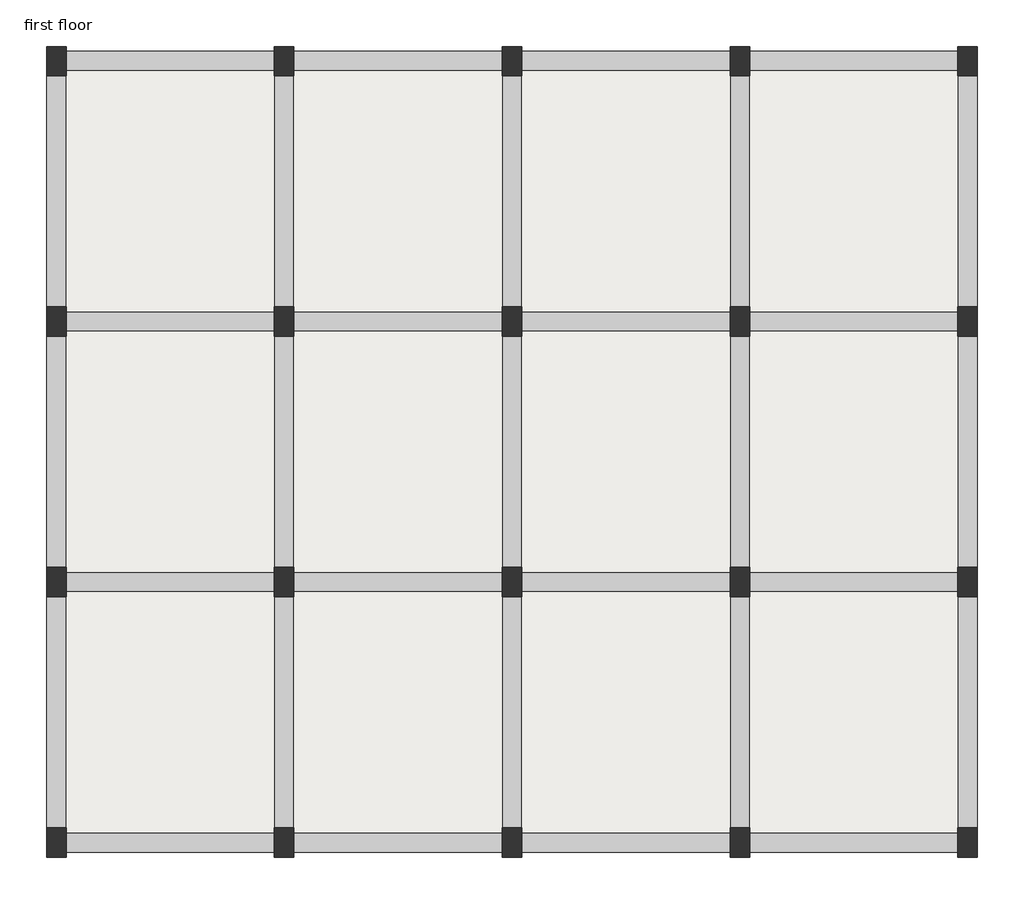
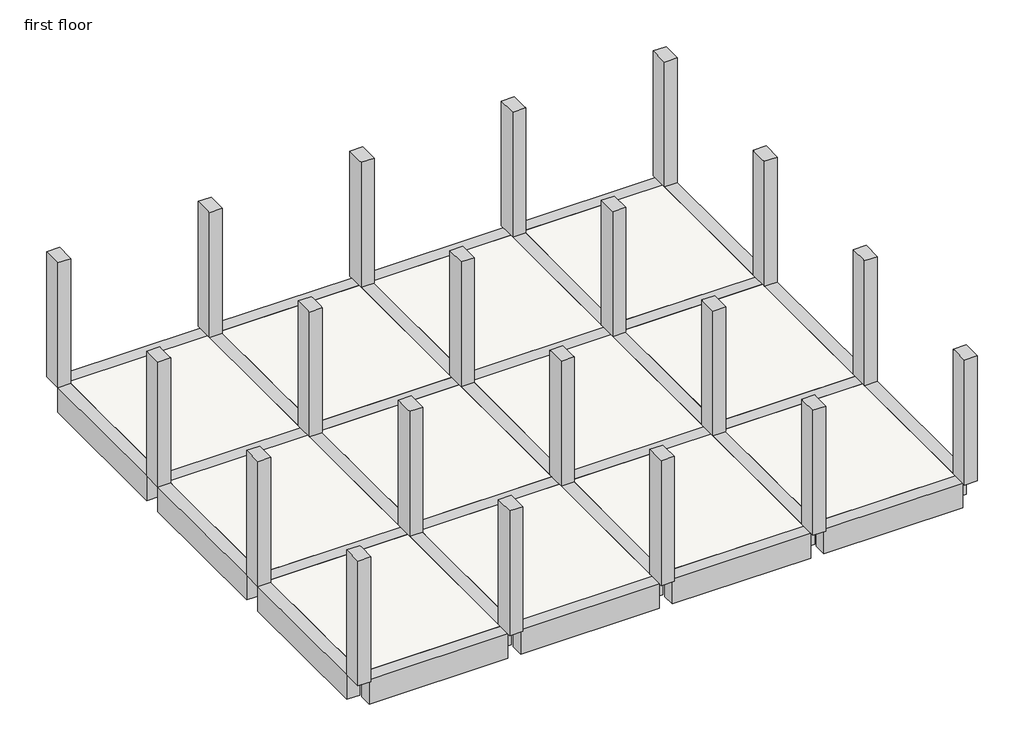
# One storey: 31 beams, 20 columns, 12 slabs.
"""IFC4 building model written with IfcOpenShell, lengths in millimetres."""

from ifc_helpers import new_model, si_unit, frame, origin, place, context, project, spatial, polyline, outline, extrude, faceted_brep, element, save

model = new_model("IFC4")

# Units and contexts
model_context = context("Model", 3, world=origin())
ifc_project = project(units=[si_unit("LENGTHUNIT", "METRE", prefix="MILLI")], contexts=[model_context])

# Site, building, storey
site = spatial("IfcSite", under=ifc_project)
building = spatial("IfcBuilding", under=site)
storey = spatial("IfcBuildingStorey", under=building, Name="first floor", Elevation=3048.0)

# Beams
placement = place(None, origin())
element("IfcBeam", 1, ObjectType="M_Concrete-Rectangular Beam : 300 x 600mm", at=placement, inside=storey, context=model_context, shape_type="SweptSolid", body=[
    extrude(outline(polyline([(-11389.0800189, 9311.4575251), (-11089.0800189, 9311.4575251), (-11089.0800189, 5761.4575251), (-11389.0800189, 5761.4575251), (-11389.0800189, 9311.4575251)])), frame((0.0, 0.0, 2448.0), z_axis=(0.0, 0.0, 1.0), x_axis=(1.0, 0.0, 0.0)), (0.0, 0.0, 1.0), 600.0),
])
element("IfcBeam", 2, ObjectType="M_Concrete-Rectangular Beam : 300 x 600mm", at=placement, inside=storey, context=model_context, shape_type="SweptSolid", body=[
    extrude(outline(polyline([(-11389.0800189, 13311.4575251), (-11089.0800189, 13311.4575251), (-11089.0800189, 9761.4575251), (-11389.0800189, 9761.4575251), (-11389.0800189, 13311.4575251)])), frame((0.0, 0.0, 2448.0), z_axis=(0.0, 0.0, 1.0), x_axis=(1.0, 0.0, 0.0)), (0.0, 0.0, 1.0), 600.0),
])
element("IfcBeam", 3, ObjectType="M_Concrete-Rectangular Beam : 300 x 600mm", at=placement, inside=storey, context=model_context, shape_type="SweptSolid", body=[
    extrude(outline(polyline([(-11389.0800189, 17311.4575251), (-11089.0800189, 17311.4575251), (-11089.0800189, 13761.4575251), (-11389.0800189, 13761.4575251), (-11389.0800189, 17311.4575251)])), frame((0.0, 0.0, 2448.0), z_axis=(0.0, 0.0, 1.0), x_axis=(1.0, 0.0, 0.0)), (0.0, 0.0, 1.0), 600.0),
])
element("IfcBeam", 4, ObjectType="M_Concrete-Rectangular Beam : 300 x 600mm", at=placement, inside=storey, context=model_context, shape_type="SweptSolid", body=[
    extrude(outline(polyline([(-7889.0800189, 9311.4575251), (-7589.0800189, 9311.4575251), (-7589.0800189, 5761.4575251), (-7889.0800189, 5761.4575251), (-7889.0800189, 9311.4575251)])), frame((0.0, 0.0, 2448.0), z_axis=(0.0, 0.0, 1.0), x_axis=(1.0, 0.0, 0.0)), (0.0, 0.0, 1.0), 600.0),
])
element("IfcBeam", 5, ObjectType="M_Concrete-Rectangular Beam : 300 x 600mm", at=placement, inside=storey, context=model_context, shape_type="SweptSolid", body=[
    extrude(outline(polyline([(-7889.0800189, 13311.4575251), (-7589.0800189, 13311.4575251), (-7589.0800189, 9761.4575251), (-7889.0800189, 9761.4575251), (-7889.0800189, 13311.4575251)])), frame((0.0, 0.0, 2448.0), z_axis=(0.0, 0.0, 1.0), x_axis=(1.0, 0.0, 0.0)), (0.0, 0.0, 1.0), 600.0),
])
element("IfcBeam", 6, ObjectType="M_Concrete-Rectangular Beam : 300 x 600mm", at=placement, inside=storey, context=model_context, shape_type="SweptSolid", body=[
    extrude(outline(polyline([(-7889.0800189, 17311.4575251), (-7589.0800189, 17311.4575251), (-7589.0800189, 13761.4575251), (-7889.0800189, 13761.4575251), (-7889.0800189, 17311.4575251)])), frame((0.0, 0.0, 2448.0), z_axis=(0.0, 0.0, 1.0), x_axis=(1.0, 0.0, 0.0)), (0.0, 0.0, 1.0), 600.0),
])
element("IfcBeam", 7, ObjectType="M_Concrete-Rectangular Beam : 300 x 600mm", at=placement, inside=storey, context=model_context, shape_type="SweptSolid", body=[
    extrude(outline(polyline([(-4389.0800189, 9311.4575251), (-4089.0800189, 9311.4575251), (-4089.0800189, 5761.4575251), (-4389.0800189, 5761.4575251), (-4389.0800189, 9311.4575251)])), frame((0.0, 0.0, 2448.0), z_axis=(0.0, 0.0, 1.0), x_axis=(1.0, 0.0, 0.0)), (0.0, 0.0, 1.0), 600.0),
])
element("IfcBeam", 8, ObjectType="M_Concrete-Rectangular Beam : 300 x 600mm", at=placement, inside=storey, context=model_context, shape_type="SweptSolid", body=[
    extrude(outline(polyline([(-4389.0800189, 13311.4575251), (-4089.0800189, 13311.4575251), (-4089.0800189, 9761.4575251), (-4389.0800189, 9761.4575251), (-4389.0800189, 13311.4575251)])), frame((0.0, 0.0, 2448.0), z_axis=(0.0, 0.0, 1.0), x_axis=(1.0, 0.0, 0.0)), (0.0, 0.0, 1.0), 600.0),
])
element("IfcBeam", 9, ObjectType="M_Concrete-Rectangular Beam : 300 x 600mm", at=placement, inside=storey, context=model_context, shape_type="SweptSolid", body=[
    extrude(outline(polyline([(-4389.0800189, 17311.4575251), (-4089.0800189, 17311.4575251), (-4089.0800189, 13761.4575251), (-4389.0800189, 13761.4575251), (-4389.0800189, 17311.4575251)])), frame((0.0, 0.0, 2448.0), z_axis=(0.0, 0.0, 1.0), x_axis=(1.0, 0.0, 0.0)), (0.0, 0.0, 1.0), 600.0),
])
element("IfcBeam", 10, ObjectType="M_Concrete-Rectangular Beam : 300 x 600mm", at=placement, inside=storey, context=model_context, shape_type="SweptSolid", body=[
    extrude(outline(polyline([(-889.0800189, 9311.4575251), (-589.0800189, 9311.4575251), (-589.0800189, 5761.4575251), (-889.0800189, 5761.4575251), (-889.0800189, 9311.4575251)])), frame((0.0, 0.0, 2448.0), z_axis=(0.0, 0.0, 1.0), x_axis=(1.0, 0.0, 0.0)), (0.0, 0.0, 1.0), 600.0),
])
element("IfcBeam", 11, ObjectType="M_Concrete-Rectangular Beam : 300 x 600mm", at=placement, inside=storey, context=model_context, shape_type="SweptSolid", body=[
    extrude(outline(polyline([(-889.0800189, 13311.4575251), (-589.0800189, 13311.4575251), (-589.0800189, 9761.4575251), (-889.0800189, 9761.4575251), (-889.0800189, 13311.4575251)])), frame((0.0, 0.0, 2448.0), z_axis=(0.0, 0.0, 1.0), x_axis=(1.0, 0.0, 0.0)), (0.0, 0.0, 1.0), 600.0),
])
element("IfcBeam", 12, ObjectType="M_Concrete-Rectangular Beam : 300 x 600mm", at=placement, inside=storey, context=model_context, shape_type="SweptSolid", body=[
    extrude(outline(polyline([(-889.0800189, 17311.4575251), (-589.0800189, 17311.4575251), (-589.0800189, 13761.4575251), (-889.0800189, 13761.4575251), (-889.0800189, 17311.4575251)])), frame((0.0, 0.0, 2448.0), z_axis=(0.0, 0.0, 1.0), x_axis=(1.0, 0.0, 0.0)), (0.0, 0.0, 1.0), 600.0),
])
element("IfcBeam", 13, ObjectType="M_Concrete-Rectangular Beam : 300 x 600mm", at=placement, inside=storey, context=model_context, shape_type="SweptSolid", body=[
    extrude(outline(polyline([(2610.9199811, 9311.4575251), (2910.9199811, 9311.4575251), (2910.9199811, 5761.4575251), (2610.9199811, 5761.4575251), (2610.9199811, 9311.4575251)])), frame((0.0, 0.0, 2448.0), z_axis=(0.0, 0.0, 1.0), x_axis=(1.0, 0.0, 0.0)), (0.0, 0.0, 1.0), 600.0),
])
element("IfcBeam", 14, ObjectType="M_Concrete-Rectangular Beam : 300 x 600mm", at=placement, inside=storey, context=model_context, shape_type="SweptSolid", body=[
    extrude(outline(polyline([(2610.9199811, 13311.4575251), (2910.9199811, 13311.4575251), (2910.9199811, 9761.4575251), (2610.9199811, 9761.4575251), (2610.9199811, 13311.4575251)])), frame((0.0, 0.0, 2448.0), z_axis=(0.0, 0.0, 1.0), x_axis=(1.0, 0.0, 0.0)), (0.0, 0.0, 1.0), 600.0),
])
element("IfcBeam", 15, ObjectType="M_Concrete-Rectangular Beam : 300 x 600mm", at=placement, inside=storey, context=model_context, shape_type="SweptSolid", body=[
    extrude(outline(polyline([(2610.9199811, 17311.4575251), (2910.9199811, 17311.4575251), (2910.9199811, 13761.4575251), (2610.9199811, 13761.4575251), (2610.9199811, 17311.4575251)])), frame((0.0, 0.0, 2448.0), z_axis=(0.0, 0.0, 1.0), x_axis=(1.0, 0.0, 0.0)), (0.0, 0.0, 1.0), 600.0),
])
element("IfcBeam", 16, ObjectType="M_Concrete-Rectangular Beam : 300 x 600mm", at=placement, inside=storey, context=model_context, shape_type="Brep", body=[
    faceted_brep([(-11089.0800189, 17386.4575251, 3048.0), (-7889.0800189, 17386.4575251, 3048.0), (-7889.0800189, 17686.4575251, 3048.0), (-11089.0800189, 17686.4575251, 3048.0), (-11089.0800189, 17386.4575251, 2748.0), (-11089.0800189, 17386.4575251, 2448.0), (-7889.0800189, 17386.4575251, 2448.0), (-7889.0800189, 17386.4575251, 2748.0), (-7889.0800189, 17686.4575251, 2448.0), (-11089.0800189, 17686.4575251, 2448.0)], [[[0, 1, 2, 3]], [[0, 4, 5, 6, 7, 1]], [[8, 6, 5, 9]], [[9, 3, 2, 8]], [[5, 4, 0, 3, 9]], [[1, 7, 6, 8, 2]]]),
])
element("IfcBeam", 17, ObjectType="M_Concrete-Rectangular Beam : 300 x 600mm", at=placement, inside=storey, context=model_context, shape_type="Brep", body=[
    faceted_brep([(-7589.0800189, 17386.4575251, 3048.0), (-4389.0800189, 17386.4575251, 3048.0), (-4389.0800189, 17686.4575251, 3048.0), (-7589.0800189, 17686.4575251, 3048.0), (-7589.0800189, 17386.4575251, 2748.0), (-7589.0800189, 17386.4575251, 2448.0), (-4389.0800189, 17386.4575251, 2448.0), (-4389.0800189, 17386.4575251, 2748.0), (-4389.0800189, 17686.4575251, 2448.0), (-7589.0800189, 17686.4575251, 2448.0)], [[[0, 1, 2, 3]], [[0, 4, 5, 6, 7, 1]], [[8, 6, 5, 9]], [[9, 3, 2, 8]], [[5, 4, 0, 3, 9]], [[1, 7, 6, 8, 2]]]),
])
element("IfcBeam", 18, ObjectType="M_Concrete-Rectangular Beam : 300 x 600mm", at=placement, inside=storey, context=model_context, shape_type="Brep", body=[
    faceted_brep([(-4089.0800189, 17386.4575251, 3048.0), (-889.0800189, 17386.4575251, 3048.0), (-889.0800189, 17686.4575251, 3048.0), (-4089.0800189, 17686.4575251, 3048.0), (-4089.0800189, 17386.4575251, 2748.0), (-4089.0800189, 17386.4575251, 2448.0), (-889.0800189, 17386.4575251, 2448.0), (-889.0800189, 17386.4575251, 2748.0), (-889.0800189, 17686.4575251, 2448.0), (-4089.0800189, 17686.4575251, 2448.0)], [[[0, 1, 2, 3]], [[0, 4, 5, 6, 7, 1]], [[8, 6, 5, 9]], [[9, 3, 2, 8]], [[5, 4, 0, 3, 9]], [[1, 7, 6, 8, 2]]]),
])
element("IfcBeam", 19, ObjectType="M_Concrete-Rectangular Beam : 300 x 600mm", at=placement, inside=storey, context=model_context, shape_type="Brep", body=[
    faceted_brep([(-589.0800189, 17386.4575251, 3048.0), (2610.9199811, 17386.4575251, 3048.0), (2610.9199811, 17686.4575251, 3048.0), (-589.0800189, 17686.4575251, 3048.0), (-589.0800189, 17386.4575251, 2748.0), (-589.0800189, 17386.4575251, 2448.0), (2610.9199811, 17386.4575251, 2448.0), (2610.9199811, 17386.4575251, 2748.0), (2610.9199811, 17686.4575251, 2448.0), (-589.0800189, 17686.4575251, 2448.0)], [[[0, 1, 2, 3]], [[0, 4, 5, 6, 7, 1]], [[8, 6, 5, 9]], [[9, 3, 2, 8]], [[5, 4, 0, 3, 9]], [[1, 7, 6, 8, 2]]]),
])
element("IfcBeam", 20, ObjectType="M_Concrete-Rectangular Beam : 300 x 600mm", at=placement, inside=storey, context=model_context, shape_type="Brep", body=[
    faceted_brep([(-11089.0800189, 13386.4575251, 3048.0), (-7889.0800189, 13386.4575251, 3048.0), (-7889.0800189, 13686.4575251, 3048.0), (-11089.0800189, 13686.4575251, 3048.0), (-11089.0800189, 13386.4575251, 2748.0), (-11089.0800189, 13386.4575251, 2448.0), (-7889.0800189, 13386.4575251, 2448.0), (-7889.0800189, 13386.4575251, 2748.0), (-7889.0800189, 13686.4575251, 2448.0), (-11089.0800189, 13686.4575251, 2448.0), (-11089.0800189, 13686.4575251, 2748.0), (-7889.0800189, 13686.4575251, 2748.0)], [[[0, 1, 2, 3]], [[0, 4, 5, 6, 7, 1]], [[8, 6, 5, 9]], [[9, 10, 3, 2, 11, 8]], [[5, 4, 0, 3, 10, 9]], [[1, 7, 6, 8, 11, 2]]]),
])
element("IfcBeam", 21, ObjectType="M_Concrete-Rectangular Beam : 300 x 600mm", at=placement, inside=storey, context=model_context, shape_type="Brep", body=[
    faceted_brep([(-7589.0800189, 13686.4575251, 3048.0), (-7589.0800189, 13386.4575251, 3048.0), (-4389.0800189, 13386.4575251, 3048.0), (-4389.0800189, 13686.4575251, 3048.0), (-7589.0800189, 13386.4575251, 2748.0), (-7589.0800189, 13386.4575251, 2448.0), (-4389.0800189, 13386.4575251, 2448.0), (-4389.0800189, 13386.4575251, 2748.0), (-7589.0800189, 13686.4575251, 2448.0), (-4389.0800189, 13686.4575251, 2448.0), (-7589.0800189, 13686.4575251, 2748.0), (-4389.0800189, 13686.4575251, 2748.0)], [[[0, 1, 2, 3]], [[1, 4, 5, 6, 7, 2]], [[5, 8, 9, 6]], [[8, 10, 0, 3, 11, 9]], [[5, 4, 1, 0, 10, 8]], [[2, 7, 6, 9, 11, 3]]]),
])
element("IfcBeam", 22, ObjectType="M_Concrete-Rectangular Beam : 300 x 600mm", at=placement, inside=storey, context=model_context, shape_type="Brep", body=[
    faceted_brep([(-4089.0800189, 13686.4575251, 3048.0), (-4089.0800189, 13386.4575251, 3048.0), (-889.0800189, 13386.4575251, 3048.0), (-889.0800189, 13686.4575251, 3048.0), (-4089.0800189, 13386.4575251, 2748.0), (-4089.0800189, 13386.4575251, 2448.0), (-889.0800189, 13386.4575251, 2448.0), (-889.0800189, 13386.4575251, 2748.0), (-4089.0800189, 13686.4575251, 2448.0), (-889.0800189, 13686.4575251, 2448.0), (-4089.0800189, 13686.4575251, 2748.0), (-889.0800189, 13686.4575251, 2748.0)], [[[0, 1, 2, 3]], [[1, 4, 5, 6, 7, 2]], [[5, 8, 9, 6]], [[8, 10, 0, 3, 11, 9]], [[5, 4, 1, 0, 10, 8]], [[2, 7, 6, 9, 11, 3]]]),
])
element("IfcBeam", 23, ObjectType="M_Concrete-Rectangular Beam : 300 x 600mm", at=placement, inside=storey, context=model_context, shape_type="Brep", body=[
    faceted_brep([(-589.0800189, 13686.4575251, 3048.0), (-589.0800189, 13386.4575251, 3048.0), (2610.9199811, 13386.4575251, 3048.0), (2610.9199811, 13686.4575251, 3048.0), (-589.0800189, 13386.4575251, 2748.0), (-589.0800189, 13386.4575251, 2448.0), (2610.9199811, 13386.4575251, 2448.0), (2610.9199811, 13386.4575251, 2748.0), (-589.0800189, 13686.4575251, 2448.0), (2610.9199811, 13686.4575251, 2448.0), (-589.0800189, 13686.4575251, 2748.0), (2610.9199811, 13686.4575251, 2748.0)], [[[0, 1, 2, 3]], [[1, 4, 5, 6, 7, 2]], [[5, 8, 9, 6]], [[8, 10, 0, 3, 11, 9]], [[5, 4, 1, 0, 10, 8]], [[2, 7, 6, 9, 11, 3]]]),
])
element("IfcBeam", 24, ObjectType="M_Concrete-Rectangular Beam : 300 x 600mm", at=placement, inside=storey, context=model_context, shape_type="Brep", body=[
    faceted_brep([(-11089.0800189, 9386.4575251, 3048.0), (-7889.0800189, 9386.4575251, 3048.0), (-7889.0800189, 9686.4575251, 3048.0), (-11089.0800189, 9686.4575251, 3048.0), (-11089.0800189, 9386.4575251, 2748.0), (-11089.0800189, 9386.4575251, 2448.0), (-7889.0800189, 9386.4575251, 2448.0), (-7889.0800189, 9386.4575251, 2748.0), (-7889.0800189, 9686.4575251, 2448.0), (-11089.0800189, 9686.4575251, 2448.0), (-11089.0800189, 9686.4575251, 2748.0), (-7889.0800189, 9686.4575251, 2748.0)], [[[0, 1, 2, 3]], [[0, 4, 5, 6, 7, 1]], [[8, 6, 5, 9]], [[9, 10, 3, 2, 11, 8]], [[5, 4, 0, 3, 10, 9]], [[1, 7, 6, 8, 11, 2]]]),
])
element("IfcBeam", 25, ObjectType="M_Concrete-Rectangular Beam : 300 x 600mm", at=placement, inside=storey, context=model_context, shape_type="Brep", body=[
    faceted_brep([(-7589.0800189, 9686.4575251, 3048.0), (-7589.0800189, 9386.4575251, 3048.0), (-4389.0800189, 9386.4575251, 3048.0), (-4389.0800189, 9686.4575251, 3048.0), (-7589.0800189, 9386.4575251, 2748.0), (-7589.0800189, 9386.4575251, 2448.0), (-4389.0800189, 9386.4575251, 2448.0), (-4389.0800189, 9386.4575251, 2748.0), (-7589.0800189, 9686.4575251, 2448.0), (-4389.0800189, 9686.4575251, 2448.0), (-7589.0800189, 9686.4575251, 2748.0), (-4389.0800189, 9686.4575251, 2748.0)], [[[0, 1, 2, 3]], [[1, 4, 5, 6, 7, 2]], [[5, 8, 9, 6]], [[8, 10, 0, 3, 11, 9]], [[5, 4, 1, 0, 10, 8]], [[2, 7, 6, 9, 11, 3]]]),
])
element("IfcBeam", 26, ObjectType="M_Concrete-Rectangular Beam : 300 x 600mm", at=placement, inside=storey, context=model_context, shape_type="Brep", body=[
    faceted_brep([(-4089.0800189, 9686.4575251, 3048.0), (-4089.0800189, 9386.4575251, 3048.0), (-889.0800189, 9386.4575251, 3048.0), (-889.0800189, 9686.4575251, 3048.0), (-4089.0800189, 9386.4575251, 2748.0), (-4089.0800189, 9386.4575251, 2448.0), (-889.0800189, 9386.4575251, 2448.0), (-889.0800189, 9386.4575251, 2748.0), (-4089.0800189, 9686.4575251, 2448.0), (-889.0800189, 9686.4575251, 2448.0), (-4089.0800189, 9686.4575251, 2748.0), (-889.0800189, 9686.4575251, 2748.0)], [[[0, 1, 2, 3]], [[1, 4, 5, 6, 7, 2]], [[5, 8, 9, 6]], [[8, 10, 0, 3, 11, 9]], [[5, 4, 1, 0, 10, 8]], [[2, 7, 6, 9, 11, 3]]]),
])
element("IfcBeam", 27, ObjectType="M_Concrete-Rectangular Beam : 300 x 600mm", at=placement, inside=storey, context=model_context, shape_type="Brep", body=[
    faceted_brep([(-589.0800189, 9686.4575251, 3048.0), (-589.0800189, 9386.4575251, 3048.0), (2610.9199811, 9386.4575251, 3048.0), (2610.9199811, 9686.4575251, 3048.0), (-589.0800189, 9386.4575251, 2748.0), (-589.0800189, 9386.4575251, 2448.0), (2610.9199811, 9386.4575251, 2448.0), (2610.9199811, 9386.4575251, 2748.0), (-589.0800189, 9686.4575251, 2448.0), (2610.9199811, 9686.4575251, 2448.0), (-589.0800189, 9686.4575251, 2748.0), (2610.9199811, 9686.4575251, 2748.0)], [[[0, 1, 2, 3]], [[1, 4, 5, 6, 7, 2]], [[5, 8, 9, 6]], [[8, 10, 0, 3, 11, 9]], [[5, 4, 1, 0, 10, 8]], [[2, 7, 6, 9, 11, 3]]]),
])
element("IfcBeam", 28, ObjectType="M_Concrete-Rectangular Beam : 300 x 600mm", at=placement, inside=storey, context=model_context, shape_type="Brep", body=[
    faceted_brep([(-7889.0800189, 5386.4575251, 3048.0), (-7889.0800189, 5686.4575251, 3048.0), (-11089.0800189, 5686.4575251, 3048.0), (-11089.0800189, 5386.4575251, 3048.0), (-11089.0800189, 5386.4575251, 2448.0), (-7889.0800189, 5386.4575251, 2448.0), (-11089.0800189, 5686.4575251, 2448.0), (-7889.0800189, 5686.4575251, 2448.0), (-11089.0800189, 5686.4575251, 2748.0), (-7889.0800189, 5686.4575251, 2748.0)], [[[0, 1, 2, 3]], [[3, 4, 5, 0]], [[6, 7, 5, 4]], [[6, 8, 2, 1, 9, 7]], [[2, 8, 6, 4, 3]], [[0, 5, 7, 9, 1]]]),
])
element("IfcBeam", 29, ObjectType="M_Concrete-Rectangular Beam : 300 x 600mm", at=placement, inside=storey, context=model_context, shape_type="Brep", body=[
    faceted_brep([(-4389.0800189, 5386.4575251, 3048.0), (-4389.0800189, 5686.4575251, 3048.0), (-7589.0800189, 5686.4575251, 3048.0), (-7589.0800189, 5386.4575251, 3048.0), (-7589.0800189, 5386.4575251, 2448.0), (-4389.0800189, 5386.4575251, 2448.0), (-7589.0800189, 5686.4575251, 2448.0), (-4389.0800189, 5686.4575251, 2448.0), (-7589.0800189, 5686.4575251, 2748.0), (-4389.0800189, 5686.4575251, 2748.0)], [[[0, 1, 2, 3]], [[3, 4, 5, 0]], [[6, 7, 5, 4]], [[6, 8, 2, 1, 9, 7]], [[2, 8, 6, 4, 3]], [[0, 5, 7, 9, 1]]]),
])
element("IfcBeam", 30, ObjectType="M_Concrete-Rectangular Beam : 300 x 600mm", at=placement, inside=storey, context=model_context, shape_type="Brep", body=[
    faceted_brep([(-889.0800189, 5386.4575251, 3048.0), (-889.0800189, 5686.4575251, 3048.0), (-4089.0800189, 5686.4575251, 3048.0), (-4089.0800189, 5386.4575251, 3048.0), (-4089.0800189, 5386.4575251, 2448.0), (-889.0800189, 5386.4575251, 2448.0), (-4089.0800189, 5686.4575251, 2448.0), (-889.0800189, 5686.4575251, 2448.0), (-4089.0800189, 5686.4575251, 2748.0), (-889.0800189, 5686.4575251, 2748.0)], [[[0, 1, 2, 3]], [[3, 4, 5, 0]], [[6, 7, 5, 4]], [[6, 8, 2, 1, 9, 7]], [[2, 8, 6, 4, 3]], [[0, 5, 7, 9, 1]]]),
])
element("IfcBeam", 31, ObjectType="M_Concrete-Rectangular Beam : 300 x 600mm", at=placement, inside=storey, context=model_context, shape_type="Brep", body=[
    faceted_brep([(2610.9199811, 5386.4575251, 3048.0), (2610.9199811, 5686.4575251, 3048.0), (-589.0800189, 5686.4575251, 3048.0), (-589.0800189, 5386.4575251, 3048.0), (-589.0800189, 5386.4575251, 2448.0), (2610.9199811, 5386.4575251, 2448.0), (-589.0800189, 5686.4575251, 2448.0), (2610.9199811, 5686.4575251, 2448.0), (-589.0800189, 5686.4575251, 2748.0), (2610.9199811, 5686.4575251, 2748.0)], [[[0, 1, 2, 3]], [[3, 4, 5, 0]], [[6, 7, 5, 4]], [[6, 8, 2, 1, 9, 7]], [[2, 8, 6, 4, 3]], [[0, 5, 7, 9, 1]]]),
])

# Columns
element("IfcColumn", 32, ObjectType="M_Concrete-Rectangular-Column : 300 x 450mm", at=placement, inside=storey, context=model_context, shape_type="Brep", body=[
    faceted_brep([(-11089.0800189, 17761.4575251, 3048.0), (-11089.0800189, 17311.4575251, 3048.0), (-11389.0800189, 17311.4575251, 3048.0), (-11389.0800189, 17761.4575251, 3048.0), (-11089.0800189, 17761.4575251, 6096.0), (-11089.0800189, 17386.4575251, 6096.0), (-11089.0800189, 17311.4575251, 6096.0), (-11389.0800189, 17311.4575251, 6096.0), (-11389.0800189, 17761.4575251, 6096.0)], [[[0, 1, 2, 3]], [[4, 5, 6, 1, 0]], [[6, 7, 2, 1]], [[7, 8, 3, 2]], [[8, 4, 0, 3]], [[4, 8, 7, 6, 5]]]),
])
element("IfcColumn", 33, ObjectType="M_Concrete-Rectangular-Column : 300 x 450mm", at=placement, inside=storey, context=model_context, shape_type="Brep", body=[
    faceted_brep([(-11089.0800189, 13761.4575251, 3048.0), (-11089.0800189, 13311.4575251, 3048.0), (-11389.0800189, 13311.4575251, 3048.0), (-11389.0800189, 13761.4575251, 3048.0), (-11089.0800189, 13761.4575251, 6096.0), (-11089.0800189, 13686.4575251, 6096.0), (-11089.0800189, 13386.4575251, 6096.0), (-11089.0800189, 13311.4575251, 6096.0), (-11389.0800189, 13311.4575251, 6096.0), (-11389.0800189, 13761.4575251, 6096.0)], [[[0, 1, 2, 3]], [[4, 5, 6, 7, 1, 0]], [[7, 8, 2, 1]], [[8, 9, 3, 2]], [[9, 4, 0, 3]], [[4, 9, 8, 7, 6, 5]]]),
])
element("IfcColumn", 34, ObjectType="M_Concrete-Rectangular-Column : 300 x 450mm", at=placement, inside=storey, context=model_context, shape_type="Brep", body=[
    faceted_brep([(-11089.0800189, 9761.4575251, 3048.0), (-11089.0800189, 9311.4575251, 3048.0), (-11389.0800189, 9311.4575251, 3048.0), (-11389.0800189, 9761.4575251, 3048.0), (-11089.0800189, 9761.4575251, 6096.0), (-11089.0800189, 9686.4575251, 6096.0), (-11089.0800189, 9386.4575251, 6096.0), (-11089.0800189, 9311.4575251, 6096.0), (-11389.0800189, 9311.4575251, 6096.0), (-11389.0800189, 9761.4575251, 6096.0)], [[[0, 1, 2, 3]], [[4, 5, 6, 7, 1, 0]], [[7, 8, 2, 1]], [[8, 9, 3, 2]], [[9, 4, 0, 3]], [[4, 9, 8, 7, 6, 5]]]),
])
element("IfcColumn", 35, ObjectType="M_Concrete-Rectangular-Column : 300 x 450mm", at=placement, inside=storey, context=model_context, shape_type="Brep", body=[
    faceted_brep([(-11089.0800189, 5761.4575251, 3048.0), (-11089.0800189, 5311.4575251, 3048.0), (-11389.0800189, 5311.4575251, 3048.0), (-11389.0800189, 5761.4575251, 3048.0), (-11089.0800189, 5761.4575251, 6096.0), (-11089.0800189, 5686.4575251, 6096.0), (-11089.0800189, 5311.4575251, 6096.0), (-11389.0800189, 5311.4575251, 6096.0), (-11389.0800189, 5761.4575251, 6096.0)], [[[0, 1, 2, 3]], [[4, 5, 6, 1, 0]], [[6, 7, 2, 1]], [[7, 8, 3, 2]], [[8, 4, 0, 3]], [[4, 8, 7, 6, 5]]]),
])
element("IfcColumn", 36, ObjectType="M_Concrete-Rectangular-Column : 300 x 450mm", at=placement, inside=storey, context=model_context, shape_type="Brep", body=[
    faceted_brep([(-7589.0800189, 17761.4575251, 3048.0), (-7589.0800189, 17311.4575251, 3048.0), (-7889.0800189, 17311.4575251, 3048.0), (-7889.0800189, 17761.4575251, 3048.0), (-7589.0800189, 17761.4575251, 6096.0), (-7589.0800189, 17386.4575251, 6096.0), (-7589.0800189, 17311.4575251, 6096.0), (-7889.0800189, 17311.4575251, 6096.0), (-7889.0800189, 17386.4575251, 6096.0), (-7889.0800189, 17761.4575251, 6096.0)], [[[0, 1, 2, 3]], [[4, 5, 6, 1, 0]], [[6, 7, 2, 1]], [[7, 8, 9, 3, 2]], [[9, 4, 0, 3]], [[4, 9, 8, 7, 6, 5]]]),
])
element("IfcColumn", 37, ObjectType="M_Concrete-Rectangular-Column : 300 x 450mm", at=placement, inside=storey, context=model_context, shape_type="Brep", body=[
    faceted_brep([(-7589.0800189, 13761.4575251, 3048.0), (-7589.0800189, 13311.4575251, 3048.0), (-7889.0800189, 13311.4575251, 3048.0), (-7889.0800189, 13761.4575251, 3048.0), (-7589.0800189, 13761.4575251, 6096.0), (-7589.0800189, 13686.4575251, 6096.0), (-7589.0800189, 13386.4575251, 6096.0), (-7589.0800189, 13311.4575251, 6096.0), (-7889.0800189, 13311.4575251, 6096.0), (-7889.0800189, 13386.4575251, 6096.0), (-7889.0800189, 13686.4575251, 6096.0), (-7889.0800189, 13761.4575251, 6096.0)], [[[0, 1, 2, 3]], [[4, 5, 6, 7, 1, 0]], [[7, 8, 2, 1]], [[8, 9, 10, 11, 3, 2]], [[11, 4, 0, 3]], [[4, 11, 10, 9, 8, 7, 6, 5]]]),
])
element("IfcColumn", 38, ObjectType="M_Concrete-Rectangular-Column : 300 x 450mm", at=placement, inside=storey, context=model_context, shape_type="Brep", body=[
    faceted_brep([(-7589.0800189, 9761.4575251, 3048.0), (-7589.0800189, 9311.4575251, 3048.0), (-7889.0800189, 9311.4575251, 3048.0), (-7889.0800189, 9761.4575251, 3048.0), (-7589.0800189, 9761.4575251, 6096.0), (-7589.0800189, 9686.4575251, 6096.0), (-7589.0800189, 9386.4575251, 6096.0), (-7589.0800189, 9311.4575251, 6096.0), (-7889.0800189, 9311.4575251, 6096.0), (-7889.0800189, 9386.4575251, 6096.0), (-7889.0800189, 9686.4575251, 6096.0), (-7889.0800189, 9761.4575251, 6096.0)], [[[0, 1, 2, 3]], [[4, 5, 6, 7, 1, 0]], [[7, 8, 2, 1]], [[8, 9, 10, 11, 3, 2]], [[11, 4, 0, 3]], [[4, 11, 10, 9, 8, 7, 6, 5]]]),
])
element("IfcColumn", 39, ObjectType="M_Concrete-Rectangular-Column : 300 x 450mm", at=placement, inside=storey, context=model_context, shape_type="Brep", body=[
    faceted_brep([(-7589.0800189, 5761.4575251, 3048.0), (-7589.0800189, 5311.4575251, 3048.0), (-7889.0800189, 5311.4575251, 3048.0), (-7889.0800189, 5761.4575251, 3048.0), (-7589.0800189, 5761.4575251, 6096.0), (-7589.0800189, 5686.4575251, 6096.0), (-7589.0800189, 5311.4575251, 6096.0), (-7889.0800189, 5311.4575251, 6096.0), (-7889.0800189, 5686.4575251, 6096.0), (-7889.0800189, 5761.4575251, 6096.0)], [[[0, 1, 2, 3]], [[4, 5, 6, 1, 0]], [[6, 7, 2, 1]], [[7, 8, 9, 3, 2]], [[9, 4, 0, 3]], [[4, 9, 8, 7, 6, 5]]]),
])
element("IfcColumn", 40, ObjectType="M_Concrete-Rectangular-Column : 300 x 450mm", at=placement, inside=storey, context=model_context, shape_type="Brep", body=[
    faceted_brep([(-4089.0800189, 17761.4575251, 3048.0), (-4089.0800189, 17311.4575251, 3048.0), (-4389.0800189, 17311.4575251, 3048.0), (-4389.0800189, 17761.4575251, 3048.0), (-4089.0800189, 17761.4575251, 6096.0), (-4089.0800189, 17386.4575251, 6096.0), (-4089.0800189, 17311.4575251, 6096.0), (-4389.0800189, 17311.4575251, 6096.0), (-4389.0800189, 17386.4575251, 6096.0), (-4389.0800189, 17761.4575251, 6096.0)], [[[0, 1, 2, 3]], [[4, 5, 6, 1, 0]], [[6, 7, 2, 1]], [[7, 8, 9, 3, 2]], [[9, 4, 0, 3]], [[4, 9, 8, 7, 6, 5]]]),
])
element("IfcColumn", 41, ObjectType="M_Concrete-Rectangular-Column : 300 x 450mm", at=placement, inside=storey, context=model_context, shape_type="Brep", body=[
    faceted_brep([(-4089.0800189, 13761.4575251, 3048.0), (-4089.0800189, 13311.4575251, 3048.0), (-4389.0800189, 13311.4575251, 3048.0), (-4389.0800189, 13761.4575251, 3048.0), (-4089.0800189, 13761.4575251, 6096.0), (-4089.0800189, 13686.4575251, 6096.0), (-4089.0800189, 13386.4575251, 6096.0), (-4089.0800189, 13311.4575251, 6096.0), (-4389.0800189, 13311.4575251, 6096.0), (-4389.0800189, 13386.4575251, 6096.0), (-4389.0800189, 13686.4575251, 6096.0), (-4389.0800189, 13761.4575251, 6096.0)], [[[0, 1, 2, 3]], [[4, 5, 6, 7, 1, 0]], [[7, 8, 2, 1]], [[8, 9, 10, 11, 3, 2]], [[11, 4, 0, 3]], [[4, 11, 10, 9, 8, 7, 6, 5]]]),
])
element("IfcColumn", 42, ObjectType="M_Concrete-Rectangular-Column : 300 x 450mm", at=placement, inside=storey, context=model_context, shape_type="Brep", body=[
    faceted_brep([(-4089.0800189, 9761.4575251, 3048.0), (-4089.0800189, 9311.4575251, 3048.0), (-4389.0800189, 9311.4575251, 3048.0), (-4389.0800189, 9761.4575251, 3048.0), (-4089.0800189, 9761.4575251, 6096.0), (-4089.0800189, 9686.4575251, 6096.0), (-4089.0800189, 9386.4575251, 6096.0), (-4089.0800189, 9311.4575251, 6096.0), (-4389.0800189, 9311.4575251, 6096.0), (-4389.0800189, 9386.4575251, 6096.0), (-4389.0800189, 9686.4575251, 6096.0), (-4389.0800189, 9761.4575251, 6096.0)], [[[0, 1, 2, 3]], [[4, 5, 6, 7, 1, 0]], [[7, 8, 2, 1]], [[8, 9, 10, 11, 3, 2]], [[11, 4, 0, 3]], [[4, 11, 10, 9, 8, 7, 6, 5]]]),
])
element("IfcColumn", 43, ObjectType="M_Concrete-Rectangular-Column : 300 x 450mm", at=placement, inside=storey, context=model_context, shape_type="Brep", body=[
    faceted_brep([(-4089.0800189, 5761.4575251, 3048.0), (-4089.0800189, 5311.4575251, 3048.0), (-4389.0800189, 5311.4575251, 3048.0), (-4389.0800189, 5761.4575251, 3048.0), (-4089.0800189, 5761.4575251, 6096.0), (-4089.0800189, 5686.4575251, 6096.0), (-4089.0800189, 5311.4575251, 6096.0), (-4389.0800189, 5311.4575251, 6096.0), (-4389.0800189, 5686.4575251, 6096.0), (-4389.0800189, 5761.4575251, 6096.0)], [[[0, 1, 2, 3]], [[4, 5, 6, 1, 0]], [[6, 7, 2, 1]], [[7, 8, 9, 3, 2]], [[9, 4, 0, 3]], [[4, 9, 8, 7, 6, 5]]]),
])
element("IfcColumn", 44, ObjectType="M_Concrete-Rectangular-Column : 300 x 450mm", at=placement, inside=storey, context=model_context, shape_type="Brep", body=[
    faceted_brep([(-589.0800189, 17761.4575251, 3048.0), (-589.0800189, 17311.4575251, 3048.0), (-889.0800189, 17311.4575251, 3048.0), (-889.0800189, 17761.4575251, 3048.0), (-589.0800189, 17761.4575251, 6096.0), (-589.0800189, 17386.4575251, 6096.0), (-589.0800189, 17311.4575251, 6096.0), (-889.0800189, 17311.4575251, 6096.0), (-889.0800189, 17386.4575251, 6096.0), (-889.0800189, 17761.4575251, 6096.0)], [[[0, 1, 2, 3]], [[4, 5, 6, 1, 0]], [[6, 7, 2, 1]], [[7, 8, 9, 3, 2]], [[9, 4, 0, 3]], [[4, 9, 8, 7, 6, 5]]]),
])
element("IfcColumn", 45, ObjectType="M_Concrete-Rectangular-Column : 300 x 450mm", at=placement, inside=storey, context=model_context, shape_type="Brep", body=[
    faceted_brep([(-589.0800189, 13761.4575251, 3048.0), (-589.0800189, 13311.4575251, 3048.0), (-889.0800189, 13311.4575251, 3048.0), (-889.0800189, 13761.4575251, 3048.0), (-589.0800189, 13761.4575251, 6096.0), (-589.0800189, 13686.4575251, 6096.0), (-589.0800189, 13386.4575251, 6096.0), (-589.0800189, 13311.4575251, 6096.0), (-889.0800189, 13311.4575251, 6096.0), (-889.0800189, 13386.4575251, 6096.0), (-889.0800189, 13686.4575251, 6096.0), (-889.0800189, 13761.4575251, 6096.0)], [[[0, 1, 2, 3]], [[4, 5, 6, 7, 1, 0]], [[7, 8, 2, 1]], [[8, 9, 10, 11, 3, 2]], [[11, 4, 0, 3]], [[4, 11, 10, 9, 8, 7, 6, 5]]]),
])
element("IfcColumn", 46, ObjectType="M_Concrete-Rectangular-Column : 300 x 450mm", at=placement, inside=storey, context=model_context, shape_type="Brep", body=[
    faceted_brep([(-589.0800189, 9761.4575251, 3048.0), (-589.0800189, 9311.4575251, 3048.0), (-889.0800189, 9311.4575251, 3048.0), (-889.0800189, 9761.4575251, 3048.0), (-589.0800189, 9761.4575251, 6096.0), (-589.0800189, 9686.4575251, 6096.0), (-589.0800189, 9386.4575251, 6096.0), (-589.0800189, 9311.4575251, 6096.0), (-889.0800189, 9311.4575251, 6096.0), (-889.0800189, 9386.4575251, 6096.0), (-889.0800189, 9686.4575251, 6096.0), (-889.0800189, 9761.4575251, 6096.0)], [[[0, 1, 2, 3]], [[4, 5, 6, 7, 1, 0]], [[7, 8, 2, 1]], [[8, 9, 10, 11, 3, 2]], [[11, 4, 0, 3]], [[4, 11, 10, 9, 8, 7, 6, 5]]]),
])
element("IfcColumn", 47, ObjectType="M_Concrete-Rectangular-Column : 300 x 450mm", at=placement, inside=storey, context=model_context, shape_type="Brep", body=[
    faceted_brep([(-589.0800189, 5761.4575251, 3048.0), (-589.0800189, 5311.4575251, 3048.0), (-889.0800189, 5311.4575251, 3048.0), (-889.0800189, 5761.4575251, 3048.0), (-589.0800189, 5761.4575251, 6096.0), (-589.0800189, 5686.4575251, 6096.0), (-589.0800189, 5311.4575251, 6096.0), (-889.0800189, 5311.4575251, 6096.0), (-889.0800189, 5686.4575251, 6096.0), (-889.0800189, 5761.4575251, 6096.0)], [[[0, 1, 2, 3]], [[4, 5, 6, 1, 0]], [[6, 7, 2, 1]], [[7, 8, 9, 3, 2]], [[9, 4, 0, 3]], [[4, 9, 8, 7, 6, 5]]]),
])
element("IfcColumn", 48, ObjectType="M_Concrete-Rectangular-Column : 300 x 450mm", at=placement, inside=storey, context=model_context, shape_type="Brep", body=[
    faceted_brep([(2910.9199811, 17761.4575251, 3048.0), (2910.9199811, 17311.4575251, 3048.0), (2610.9199811, 17311.4575251, 3048.0), (2610.9199811, 17761.4575251, 3048.0), (2910.9199811, 17761.4575251, 6096.0), (2910.9199811, 17311.4575251, 6096.0), (2610.9199811, 17311.4575251, 6096.0), (2610.9199811, 17386.4575251, 6096.0), (2610.9199811, 17761.4575251, 6096.0)], [[[0, 1, 2, 3]], [[4, 5, 1, 0]], [[5, 6, 2, 1]], [[6, 7, 8, 3, 2]], [[8, 4, 0, 3]], [[4, 8, 7, 6, 5]]]),
])
element("IfcColumn", 49, ObjectType="M_Concrete-Rectangular-Column : 300 x 450mm", at=placement, inside=storey, context=model_context, shape_type="Brep", body=[
    faceted_brep([(2910.9199811, 13761.4575251, 3048.0), (2910.9199811, 13311.4575251, 3048.0), (2610.9199811, 13311.4575251, 3048.0), (2610.9199811, 13761.4575251, 3048.0), (2910.9199811, 13761.4575251, 6096.0), (2910.9199811, 13311.4575251, 6096.0), (2610.9199811, 13311.4575251, 6096.0), (2610.9199811, 13386.4575251, 6096.0), (2610.9199811, 13686.4575251, 6096.0), (2610.9199811, 13761.4575251, 6096.0)], [[[0, 1, 2, 3]], [[4, 5, 1, 0]], [[5, 6, 2, 1]], [[6, 7, 8, 9, 3, 2]], [[9, 4, 0, 3]], [[4, 9, 8, 7, 6, 5]]]),
])
element("IfcColumn", 50, ObjectType="M_Concrete-Rectangular-Column : 300 x 450mm", at=placement, inside=storey, context=model_context, shape_type="Brep", body=[
    faceted_brep([(2910.9199811, 9761.4575251, 3048.0), (2910.9199811, 9311.4575251, 3048.0), (2610.9199811, 9311.4575251, 3048.0), (2610.9199811, 9761.4575251, 3048.0), (2910.9199811, 9761.4575251, 6096.0), (2910.9199811, 9311.4575251, 6096.0), (2610.9199811, 9311.4575251, 6096.0), (2610.9199811, 9386.4575251, 6096.0), (2610.9199811, 9686.4575251, 6096.0), (2610.9199811, 9761.4575251, 6096.0)], [[[0, 1, 2, 3]], [[4, 5, 1, 0]], [[5, 6, 2, 1]], [[6, 7, 8, 9, 3, 2]], [[9, 4, 0, 3]], [[4, 9, 8, 7, 6, 5]]]),
])
element("IfcColumn", 51, ObjectType="M_Concrete-Rectangular-Column : 300 x 450mm", at=placement, inside=storey, context=model_context, shape_type="Brep", body=[
    faceted_brep([(2910.9199811, 5761.4575251, 3048.0), (2910.9199811, 5311.4575251, 3048.0), (2610.9199811, 5311.4575251, 3048.0), (2610.9199811, 5761.4575251, 3048.0), (2910.9199811, 5761.4575251, 6096.0), (2910.9199811, 5311.4575251, 6096.0), (2610.9199811, 5311.4575251, 6096.0), (2610.9199811, 5686.4575251, 6096.0), (2610.9199811, 5761.4575251, 6096.0)], [[[0, 1, 2, 3]], [[4, 5, 1, 0]], [[5, 6, 2, 1]], [[6, 7, 8, 3, 2]], [[8, 4, 0, 3]], [[4, 8, 7, 6, 5]]]),
])

# Slabs
element("IfcSlab", 52, ObjectType="Generic 300mm", at=placement, inside=storey, context=model_context, shape_type="Brep", body=[
    faceted_brep([(-7889.0800189, 17386.4575251, 2748.0), (-7889.0800189, 13686.4575251, 2748.0), (-11089.0800189, 13686.4575251, 2748.0), (-11089.0800189, 17386.4575251, 2748.0), (-7889.0800189, 17386.4575251, 3048.0), (-11089.0800189, 17386.4575251, 3048.0), (-11089.0800189, 17311.4575251, 3048.0), (-11089.0800189, 13761.4575251, 3048.0), (-11089.0800189, 13686.4575251, 3048.0), (-7889.0800189, 13686.4575251, 3048.0), (-7889.0800189, 13761.4575251, 3048.0), (-7889.0800189, 17311.4575251, 3048.0)], [[[0, 1, 2, 3]], [[4, 5, 6, 7, 8, 9, 10, 11]], [[1, 0, 4, 11, 10, 9]], [[2, 1, 9, 8]], [[3, 2, 8, 7, 6, 5]], [[0, 3, 5, 4]]]),
])
element("IfcSlab", 53, ObjectType="Generic 300mm", at=placement, inside=storey, context=model_context, shape_type="Brep", body=[
    faceted_brep([(-4389.0800189, 17386.4575251, 2748.0), (-4389.0800189, 13686.4575251, 2748.0), (-7589.0800189, 13686.4575251, 2748.0), (-7589.0800189, 17386.4575251, 2748.0), (-4389.0800189, 17386.4575251, 3048.0), (-7589.0800189, 17386.4575251, 3048.0), (-7589.0800189, 17311.4575251, 3048.0), (-7589.0800189, 13761.4575251, 3048.0), (-7589.0800189, 13686.4575251, 3048.0), (-4389.0800189, 13686.4575251, 3048.0), (-4389.0800189, 13761.4575251, 3048.0), (-4389.0800189, 17311.4575251, 3048.0)], [[[0, 1, 2, 3]], [[4, 5, 6, 7, 8, 9, 10, 11]], [[1, 0, 4, 11, 10, 9]], [[2, 1, 9, 8]], [[3, 2, 8, 7, 6, 5]], [[0, 3, 5, 4]]]),
])
element("IfcSlab", 54, ObjectType="Generic 300mm", at=placement, inside=storey, context=model_context, shape_type="Brep", body=[
    faceted_brep([(-889.0800189, 17386.4575251, 2748.0), (-889.0800189, 13686.4575251, 2748.0), (-4089.0800189, 13686.4575251, 2748.0), (-4089.0800189, 17386.4575251, 2748.0), (-889.0800189, 17386.4575251, 3048.0), (-4089.0800189, 17386.4575251, 3048.0), (-4089.0800189, 17311.4575251, 3048.0), (-4089.0800189, 13761.4575251, 3048.0), (-4089.0800189, 13686.4575251, 3048.0), (-889.0800189, 13686.4575251, 3048.0), (-889.0800189, 13761.4575251, 3048.0), (-889.0800189, 17311.4575251, 3048.0)], [[[0, 1, 2, 3]], [[4, 5, 6, 7, 8, 9, 10, 11]], [[1, 0, 4, 11, 10, 9]], [[2, 1, 9, 8]], [[3, 2, 8, 7, 6, 5]], [[0, 3, 5, 4]]]),
])
element("IfcSlab", 55, ObjectType="Generic 300mm", at=placement, inside=storey, context=model_context, shape_type="Brep", body=[
    faceted_brep([(2610.9199811, 17386.4575251, 2748.0), (2610.9199811, 13686.4575251, 2748.0), (-589.0800189, 13686.4575251, 2748.0), (-589.0800189, 17386.4575251, 2748.0), (2610.9199811, 17386.4575251, 3048.0), (-589.0800189, 17386.4575251, 3048.0), (-589.0800189, 17311.4575251, 3048.0), (-589.0800189, 13761.4575251, 3048.0), (-589.0800189, 13686.4575251, 3048.0), (2610.9199811, 13686.4575251, 3048.0), (2610.9199811, 13761.4575251, 3048.0), (2610.9199811, 17311.4575251, 3048.0)], [[[0, 1, 2, 3]], [[4, 5, 6, 7, 8, 9, 10, 11]], [[1, 0, 4, 11, 10, 9]], [[2, 1, 9, 8]], [[3, 2, 8, 7, 6, 5]], [[0, 3, 5, 4]]]),
])
element("IfcSlab", 56, ObjectType="Generic 300mm", at=placement, inside=storey, context=model_context, shape_type="Brep", body=[
    faceted_brep([(2610.9199811, 13386.4575251, 2748.0), (2610.9199811, 9686.4575251, 2748.0), (-589.0800189, 9686.4575251, 2748.0), (-589.0800189, 13386.4575251, 2748.0), (2610.9199811, 13386.4575251, 3048.0), (-589.0800189, 13386.4575251, 3048.0), (-589.0800189, 13311.4575251, 3048.0), (-589.0800189, 9761.4575251, 3048.0), (-589.0800189, 9686.4575251, 3048.0), (2610.9199811, 9686.4575251, 3048.0), (2610.9199811, 9761.4575251, 3048.0), (2610.9199811, 13311.4575251, 3048.0)], [[[0, 1, 2, 3]], [[4, 5, 6, 7, 8, 9, 10, 11]], [[1, 0, 4, 11, 10, 9]], [[2, 1, 9, 8]], [[3, 2, 8, 7, 6, 5]], [[0, 3, 5, 4]]]),
])
element("IfcSlab", 57, ObjectType="Generic 300mm", at=placement, inside=storey, context=model_context, shape_type="Brep", body=[
    faceted_brep([(2610.9199811, 9386.4575251, 2748.0), (2610.9199811, 5686.4575251, 2748.0), (-589.0800189, 5686.4575251, 2748.0), (-589.0800189, 9386.4575251, 2748.0), (2610.9199811, 9386.4575251, 3048.0), (-589.0800189, 9386.4575251, 3048.0), (-589.0800189, 9311.4575251, 3048.0), (-589.0800189, 5761.4575251, 3048.0), (-589.0800189, 5686.4575251, 3048.0), (2610.9199811, 5686.4575251, 3048.0), (2610.9199811, 5761.4575251, 3048.0), (2610.9199811, 9311.4575251, 3048.0)], [[[0, 1, 2, 3]], [[4, 5, 6, 7, 8, 9, 10, 11]], [[1, 0, 4, 11, 10, 9]], [[2, 1, 9, 8]], [[3, 2, 8, 7, 6, 5]], [[0, 3, 5, 4]]]),
])
element("IfcSlab", 58, ObjectType="Generic 300mm", at=placement, inside=storey, context=model_context, shape_type="Brep", body=[
    faceted_brep([(-889.0800189, 9386.4575251, 2748.0), (-889.0800189, 5686.4575251, 2748.0), (-4089.0800189, 5686.4575251, 2748.0), (-4089.0800189, 9386.4575251, 2748.0), (-889.0800189, 9386.4575251, 3048.0), (-4089.0800189, 9386.4575251, 3048.0), (-4089.0800189, 9311.4575251, 3048.0), (-4089.0800189, 5761.4575251, 3048.0), (-4089.0800189, 5686.4575251, 3048.0), (-889.0800189, 5686.4575251, 3048.0), (-889.0800189, 5761.4575251, 3048.0), (-889.0800189, 9311.4575251, 3048.0)], [[[0, 1, 2, 3]], [[4, 5, 6, 7, 8, 9, 10, 11]], [[1, 0, 4, 11, 10, 9]], [[2, 1, 9, 8]], [[3, 2, 8, 7, 6, 5]], [[0, 3, 5, 4]]]),
])
element("IfcSlab", 59, ObjectType="Generic 300mm", at=placement, inside=storey, context=model_context, shape_type="Brep", body=[
    faceted_brep([(-4389.0800189, 9386.4575251, 2748.0), (-4389.0800189, 5686.4575251, 2748.0), (-7589.0800189, 5686.4575251, 2748.0), (-7589.0800189, 9386.4575251, 2748.0), (-4389.0800189, 9386.4575251, 3048.0), (-7589.0800189, 9386.4575251, 3048.0), (-7589.0800189, 9311.4575251, 3048.0), (-7589.0800189, 5761.4575251, 3048.0), (-7589.0800189, 5686.4575251, 3048.0), (-4389.0800189, 5686.4575251, 3048.0), (-4389.0800189, 5761.4575251, 3048.0), (-4389.0800189, 9311.4575251, 3048.0)], [[[0, 1, 2, 3]], [[4, 5, 6, 7, 8, 9, 10, 11]], [[1, 0, 4, 11, 10, 9]], [[2, 1, 9, 8]], [[3, 2, 8, 7, 6, 5]], [[0, 3, 5, 4]]]),
])
element("IfcSlab", 60, ObjectType="Generic 300mm", at=placement, inside=storey, context=model_context, shape_type="Brep", body=[
    faceted_brep([(-7889.0800189, 9386.4575251, 2748.0), (-7889.0800189, 5686.4575251, 2748.0), (-11089.0800189, 5686.4575251, 2748.0), (-11089.0800189, 9386.4575251, 2748.0), (-7889.0800189, 9386.4575251, 3048.0), (-11089.0800189, 9386.4575251, 3048.0), (-11089.0800189, 9311.4575251, 3048.0), (-11089.0800189, 5761.4575251, 3048.0), (-11089.0800189, 5686.4575251, 3048.0), (-7889.0800189, 5686.4575251, 3048.0), (-7889.0800189, 5761.4575251, 3048.0), (-7889.0800189, 9311.4575251, 3048.0)], [[[0, 1, 2, 3]], [[4, 5, 6, 7, 8, 9, 10, 11]], [[1, 0, 4, 11, 10, 9]], [[2, 1, 9, 8]], [[3, 2, 8, 7, 6, 5]], [[0, 3, 5, 4]]]),
])
element("IfcSlab", 61, ObjectType="Generic 300mm", at=placement, inside=storey, context=model_context, shape_type="Brep", body=[
    faceted_brep([(-7889.0800189, 13386.4575251, 2748.0), (-7889.0800189, 9686.4575251, 2748.0), (-11089.0800189, 9686.4575251, 2748.0), (-11089.0800189, 13386.4575251, 2748.0), (-7889.0800189, 13386.4575251, 3048.0), (-11089.0800189, 13386.4575251, 3048.0), (-11089.0800189, 13311.4575251, 3048.0), (-11089.0800189, 9761.4575251, 3048.0), (-11089.0800189, 9686.4575251, 3048.0), (-7889.0800189, 9686.4575251, 3048.0), (-7889.0800189, 9761.4575251, 3048.0), (-7889.0800189, 13311.4575251, 3048.0)], [[[0, 1, 2, 3]], [[4, 5, 6, 7, 8, 9, 10, 11]], [[1, 0, 4, 11, 10, 9]], [[2, 1, 9, 8]], [[3, 2, 8, 7, 6, 5]], [[0, 3, 5, 4]]]),
])
element("IfcSlab", 62, ObjectType="Generic 300mm", at=placement, inside=storey, context=model_context, shape_type="Brep", body=[
    faceted_brep([(-4389.0800189, 13386.4575251, 2748.0), (-4389.0800189, 9686.4575251, 2748.0), (-7589.0800189, 9686.4575251, 2748.0), (-7589.0800189, 13386.4575251, 2748.0), (-4389.0800189, 13386.4575251, 3048.0), (-7589.0800189, 13386.4575251, 3048.0), (-7589.0800189, 13311.4575251, 3048.0), (-7589.0800189, 9761.4575251, 3048.0), (-7589.0800189, 9686.4575251, 3048.0), (-4389.0800189, 9686.4575251, 3048.0), (-4389.0800189, 9761.4575251, 3048.0), (-4389.0800189, 13311.4575251, 3048.0)], [[[0, 1, 2, 3]], [[4, 5, 6, 7, 8, 9, 10, 11]], [[1, 0, 4, 11, 10, 9]], [[2, 1, 9, 8]], [[3, 2, 8, 7, 6, 5]], [[0, 3, 5, 4]]]),
])
element("IfcSlab", 63, ObjectType="Generic 300mm", at=placement, inside=storey, context=model_context, shape_type="Brep", body=[
    faceted_brep([(-889.0800189, 13386.4575251, 2748.0), (-889.0800189, 9686.4575251, 2748.0), (-4089.0800189, 9686.4575251, 2748.0), (-4089.0800189, 13386.4575251, 2748.0), (-889.0800189, 13386.4575251, 3048.0), (-4089.0800189, 13386.4575251, 3048.0), (-4089.0800189, 13311.4575251, 3048.0), (-4089.0800189, 9761.4575251, 3048.0), (-4089.0800189, 9686.4575251, 3048.0), (-889.0800189, 9686.4575251, 3048.0), (-889.0800189, 9761.4575251, 3048.0), (-889.0800189, 13311.4575251, 3048.0)], [[[0, 1, 2, 3]], [[4, 5, 6, 7, 8, 9, 10, 11]], [[1, 0, 4, 11, 10, 9]], [[2, 1, 9, 8]], [[3, 2, 8, 7, 6, 5]], [[0, 3, 5, 4]]]),
])

save(model, "model.ifc")

# Revit data of these elements
# Type "M_Concrete-Rectangular Beam : 300 x 600mm"
#   Length [instance default] = 5' - 0"
#   b = 0' - 11.81102"
#   h = 1' - 11.62205"
#   Structural Material [instance default] = Concrete, Cast-in-Place gray
#   Assembly Code = ""
# Type "M_Concrete-Rectangular-Column : 300 x 450mm"
#   b = 0' - 11.81102"
#   h = 1' - 5.71654"
#   Structural Material [instance default] = Concrete, Cast-in-Place gray
# Type "Generic 300mm"
#   Function = 0
#   Layers, outside or top first: 0' - 11.81102" no material (function 1)
# Elements 1, 2, 3, 4, 5, 6, 7, 8, 9, 10, 11, 12, 13, 14, 15, 16, 17, 18, 19, 20, 21, 22, 23, 24, 25, 26, 27, 28, 29, 30, 31 (IfcBeam, "M_Concrete-Rectangular Beam : 300 x 600mm")
#   Phase Created = New Construction
#   Materials on its faces: "Concrete, Cast-in-Place gray"
# Elements 32, 33, 34, 35, 36, 37, 38, 39, 40, 41, 42, 43, 44, 45, 46, 47, 48, 49, 50, 51 (IfcColumn, "M_Concrete-Rectangular-Column : 300 x 450mm")
#   Structural Material = Concrete, Cast-in-Place gray
#   Phase Created = New Construction
#   Materials on its faces: "Concrete, Cast-in-Place gray"
# Elements 52, 53, 54, 55, 56, 57, 58, 59, 60, 61, 62, 63 (IfcSlab, "Generic 300mm")
#   Height Offset From Level = 0' - 0"
#   built-in parameter 1001954 = 1
#   Phase Created = New Construction
#   Materials on its faces: "Default Floor"
# Materials
#   "Concrete, Cast-in-Place gray": class "Concrete", colour RGB 192 192 192, transparency 0, Description = "Cast-in-place concrete", Cost = 0
#   "Default Floor": colour RGB 127 127 127, transparency 0, Cost = 0
